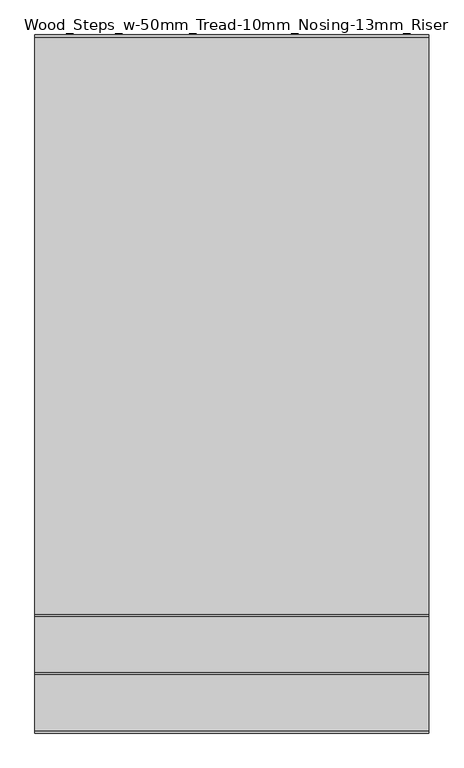
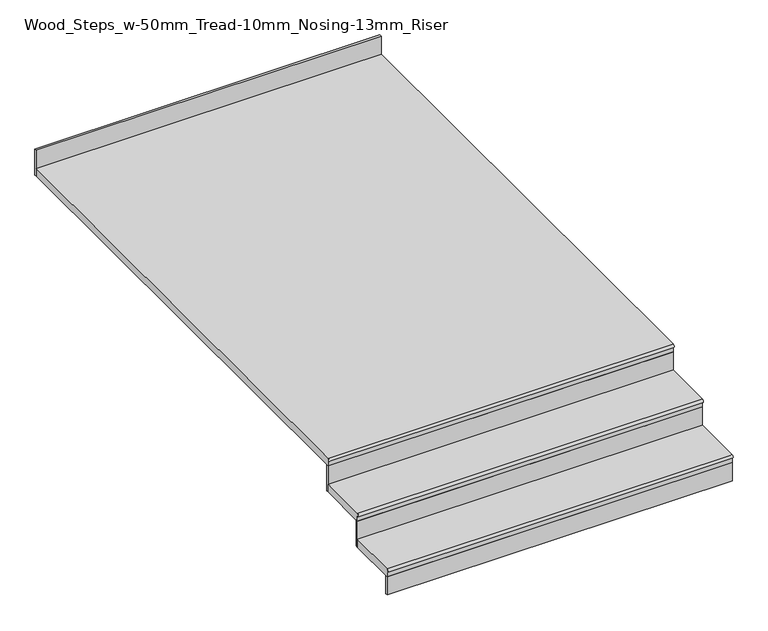
"""IFC4 building model written with IfcOpenShell, lengths in millimetres: stair flight geometry, Wood_Steps_w-50mm_Tread-10mm_Nosing-13mm_Riser."""

from ifc_helpers import new_model, si_unit, point, frame, frame_2d, origin, place, context, project, spatial, polyline, circle_curve, trimmed, segment, composite_curve, outline, extrude, source, transform, mapped, element, save


def wood_steps_w_50mm_tread_10mm_nosing_13mm_riser_5aef8f96(model_context):
    return source(origin(), model_context, "Body", "SweptSolid", [
        extrude(outline(composite_curve([segment(polyline([(1715.7806314, -261.2571429), (2025.6606314, -261.2571429), (2025.6606314, -311.2571429), (1715.7806314, -311.2571429), (1715.7806314, -281.2571429)]), True, "CONTINUOUS"), segment(trimmed(circle_curve(frame_2d((1715.7806314, -271.2571429)), 10.0), [point((1715.7806314, -281.2571429))], [point((1715.7806314, -261.2571429))], False, "CARTESIAN"), True, "CONTINUOUS")], self_intersect=False)), frame((-5125.063883, 0.0, 0.0), z_axis=(1.0, 0.0, 0.0), x_axis=(0.0, 1.0, 0.0)), (0.0, 0.0, 1.0), 2074.0134599),
        extrude(outline(polyline([(-3051.0504231, 1728.2806314), (-3051.0504231, 1715.7806314), (-5125.063883, 1715.7806314), (-5125.063883, 1728.2806314), (-3051.0504231, 1728.2806314)])), frame((0.0, 0.0, -426.72), z_axis=(0.0, 0.0, 1.0), x_axis=(1.0, 0.0, 0.0)), (0.0, 0.0, 1.0), 115.4628571),
        extrude(outline(polyline([(-3051.0504231, 2038.1606314), (-3051.0504231, 2025.6606314), (-5125.063883, 2025.6606314), (-5125.063883, 2038.1606314), (-3051.0504231, 2038.1606314)])), frame((0.0, 0.0, -311.2571429), z_axis=(0.0, 0.0, 1.0), x_axis=(1.0, 0.0, 0.0)), (0.0, 0.0, 1.0), 165.4628571),
        extrude(outline(composite_curve([segment(polyline([(2025.6606314, -95.7942857), (2330.4606314, -95.7942857), (2330.4606314, -145.7942857), (2025.6606314, -145.7942857), (2025.6606314, -115.7942857)]), True, "CONTINUOUS"), segment(trimmed(circle_curve(frame_2d((2025.6606314, -105.7942857)), 10.0), [point((2025.6606314, -115.7942857))], [point((2025.6606314, -95.7942857))], False, "CARTESIAN"), True, "CONTINUOUS")], self_intersect=False)), frame((-5125.063883, 0.0, 0.0), z_axis=(1.0, 0.0, 0.0), x_axis=(0.0, 1.0, 0.0)), (0.0, 0.0, 1.0), 2074.0134599),
        extrude(outline(polyline([(-3051.0504231, 2342.9606314), (-3051.0504231, 2330.4606314), (-5125.063883, 2330.4606314), (-5125.063883, 2342.9606314), (-3051.0504231, 2342.9606314)])), frame((0.0, 0.0, -145.7942857), z_axis=(0.0, 0.0, 1.0), x_axis=(1.0, 0.0, 0.0)), (0.0, 0.0, 1.0), 165.4628571),
        extrude(outline(polyline([(-3051.0504231, 5382.1856226), (-3051.0504231, 5369.6856226), (-5125.063883, 5369.6856226), (-5125.063883, 5382.1856226), (-3051.0504231, 5382.1856226)])), frame((0.0, 0.0, 19.6685714), z_axis=(0.0, 0.0, 1.0), x_axis=(1.0, 0.0, 0.0)), (0.0, 0.0, 1.0), 165.4628571),
        extrude(outline(composite_curve([segment(polyline([(2330.4606314, 69.6685714), (5369.6856226, 69.6685714), (5369.6856226, 19.6685714), (2330.4606314, 19.6685714), (2330.4606314, 49.6685714)]), True, "CONTINUOUS"), segment(trimmed(circle_curve(frame_2d((2330.4606314, 59.6685714)), 10.0), [point((2330.4606314, 49.6685714))], [point((2330.4606314, 69.6685714))], False, "CARTESIAN"), True, "CONTINUOUS")], self_intersect=False)), frame((-5125.063883, 0.0, 0.0), z_axis=(1.0, 0.0, 0.0), x_axis=(0.0, 1.0, 0.0)), (0.0, 0.0, 1.0), 2074.0134599),
    ])


if __name__ == "__main__":
    model = new_model("IFC4")
    model_context = context("Model", 3, world=origin())
    ifc_project = project(units=[si_unit("LENGTHUNIT", "METRE", prefix="MILLI")], contexts=[model_context])
    site = spatial("IfcSite", under=ifc_project)
    building = spatial("IfcBuilding", under=site)
    placement = place(None, origin())
    wood_steps_w_50mm_tread_10mm_nosing_13mm_riser_shape = wood_steps_w_50mm_tread_10mm_nosing_13mm_riser_5aef8f96(model_context)
    element("IfcStairFlight", 1, ObjectType="Wood_Steps_w-50mm_Tread-10mm_Nosing-13mm_Riser", at=placement, inside=building, context=model_context, shape_type="MappedRepresentation", body=[
        mapped(wood_steps_w_50mm_tread_10mm_nosing_13mm_riser_shape, transform((0.0, 0.0, 0.0), x_axis=(1.0, 0.0, 0.0), y_axis=(0.0, 1.0, 0.0), z_axis=(0.0, 0.0, 1.0))),
    ])
    save(model, "model.ifc")

# Revit data of these elements
# Element 1 (IfcStairFlight, "Wood_Steps_w-50mm_Tread-10mm_Nosing-13mm_Riser")
#   Materials on its faces: "Oak Flooring"
# Materials
#   "Oak Flooring": class "Wood", colour RGB 212 179 113, transparency 0, Description = "Quercus Rubra", Cost = 0
